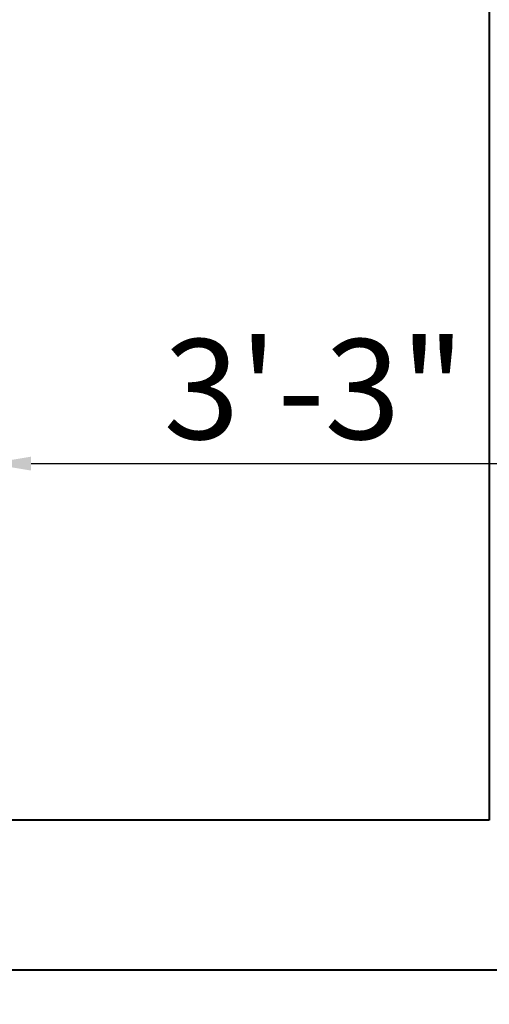
# Model space of a CAD drawing. Units: inches. Extents: x 459864 to 460310, y 324185 to 324787.
# Tile 79 of 112: x 460210 to 460238, y 324281 to 324341. Entities that reach past the tile are written whole.
import ezdxf

# ---------------------------------------------------------------- set-up
doc = ezdxf.new("R2010")
doc.units = ezdxf.units.IN
for name, color, linetype, lineweight in [('A-ANNO-DIMS', 2, 'Continuous', 18), ('A-WALL', 7, 'Continuous', 40), ('L-SITE-PATT', 252, 'Continuous', 13)]:
    doc.layers.add(name, color=color, linetype=linetype, lineweight=lineweight)
doc.styles.get("Standard").update_dxf_attribs({"font": 'arial.ttf'})
doc.dimstyles.new('ISO-25', dxfattribs={"dimtxt": 6, "dimasz": 2.5, "dimexe": 1.25, "dimexo": 0.625, "dimtad": 1, "dimdec": 1, "dimlunit": 3, "dimtxsty": 'Standard', "dimcen": 2.5, "dimadec": 0, "dimazin": 0, "dimtfac": 1, "dimtdec": 1, "dimtmove": 0, "dimatfit": 3, "dimfxl": 1, "dimarcsym": 0})

# ---------------------------------------------------------------- blocks, each defined once
blk = doc.blocks.new('*D67')
at = {"layer": 'A-ANNO-DIMS', "color": 0, "lineweight": -2, "transparency": 16777216}
for p, q in [((460208.115, 324284.108), (460208.115, 324315.133)), ((460247.115, 324284.108), (460247.115, 324315.133)), ((460210.615, 324313.883), (460244.615, 324313.883))]:
    blk.add_line(p, q, dxfattribs=at)
at = {"layer": 'A-ANNO-DIMS', "color": 0, "transparency": 16777216}
for points in [[(460210.615, 324314.3), (460210.615, 324313.467), (460208.115, 324313.883)], [(460244.615, 324314.3), (460244.615, 324313.467), (460247.115, 324313.883)]]:
    blk.add_solid(points, dxfattribs=at)
at = {"layer": 'Defpoints', "color": 0, "transparency": 16777216}
for p in [(460247.115, 324313.883), (460208.115, 324283.483), (460247.115, 324283.483)]:
    blk.add_point(p, dxfattribs=at)
at = {"layer": 'A-ANNO-DIMS', "color": 0, "transparency": 16777216, "insert": (460227.615, 324317.574), "char_height": 6, "attachment_point": 5}
blk.add_mtext('3\'-3"', dxfattribs=at)

msp = doc.modelspace()

# ---------------------------------------------------------------- hatches: boundary and pattern name
at = {"layer": 'L-SITE-PATT'}
h = msp.add_hatch(dxfattribs=at)
h.set_pattern_fill('DOTS', color=256)
h.paths.add_polyline_path([(460269.804, 324283.483), (460247.115, 324283.483), (460121.929, 324283.483), (460121.929, 324252.473), (460117.429, 324252.473), (460110.124, 324252.473), (460110.124, 324243.287), (460080.83, 324243.287), (460080.83, 324252.473), (460061.115, 324252.473), (460061.115, 324251.882), (460077.909, 324251.882), (460077.909, 324199.483), (460080.83, 324199.483), (460080.83, 324207.553), (460110.124, 324207.553), (460110.124, 324199.483), (460110.813, 324199.483), (460262.115, 324199.483), (460269.804, 324199.483)], flags=17)
edge = h.paths.add_edge_path(flags=0)
edge.add_ellipse((460222.59, 324263.813), major_axis=(-8.485, 8.485), ratio=1, start_angle=405, end_angle=495, ccw=False)
edge.add_line((460214.821, 324254.66), (460214.832, 324254.666))
edge.add_ellipse((460222.59, 324263.813), major_axis=(-8.485, 8.485), ratio=1, start_angle=405, end_angle=495, ccw=False)
edge.add_line((460210.759, 324261.781), (460210.768, 324261.787))
edge.add_ellipse((460222.59, 324263.813), major_axis=(-8.485, 8.485), ratio=1, start_angle=405, end_angle=495, ccw=False)
edge.add_ellipse((460222.59, 324263.813), major_axis=(-8.485, 8.485), ratio=1, start_angle=392.75402, end_angle=405, ccw=False)
edge.add_ellipse((460222.59, 324263.813), major_axis=(-8.485, 8.485), ratio=1, start_angle=380.93472, end_angle=392.75402, ccw=False)
edge.add_line((460211.337, 324267.985), (460211.34, 324267.985))
edge.add_ellipse((460222.59, 324263.813), major_axis=(-8.485, 8.485), ratio=1, start_angle=380.93472, end_angle=392.75402, ccw=False)
edge.add_ellipse((460222.59, 324263.813), major_axis=(-8.485, 8.485), ratio=1, start_angle=347.90152, end_angle=380.93472, ccw=False)
edge.add_ellipse((460222.59, 324263.813), major_axis=(-8.485, 8.485), ratio=1, start_angle=327.06192, end_angle=347.90152, ccw=False)
edge.add_ellipse((460222.59, 324263.813), major_axis=(-8.485, 8.485), ratio=1, start_angle=278.32464, end_angle=327.06192, ccw=False)
edge.add_line((460225.158, 324275.536), (460225.158, 324275.535))
edge.add_ellipse((460222.59, 324263.813), major_axis=(-8.485, 8.485), ratio=1, start_angle=278.32464, end_angle=327.06192, ccw=False)
edge.add_ellipse((460222.59, 324263.813), major_axis=(-8.485, 8.485), ratio=1, start_angle=260.64357, end_angle=278.32464, ccw=False)
edge.add_ellipse((460222.59, 324263.813), major_axis=(-8.485, 8.485), ratio=1, start_angle=225, end_angle=260.64357, ccw=False)
edge.add_line((460234.509, 324265.243), (460234.501, 324265.239))
edge.add_ellipse((460222.59, 324263.813), major_axis=(-8.485, 8.485), ratio=1, start_angle=225, end_angle=260.64357, ccw=False)
edge.add_ellipse((460222.59, 324263.813), major_axis=(-8.485, 8.485), ratio=1, start_angle=495, end_angle=585, ccw=False)
edge.add_line((460234.437, 324261.861), (460234.424, 324261.858))
edge.add_ellipse((460222.59, 324263.813), major_axis=(-8.485, 8.485), ratio=1, start_angle=495, end_angle=585, ccw=False)
edge.add_line((460227.95, 324253.067), (460227.946, 324253.083))
edge.add_ellipse((460222.59, 324263.813), major_axis=(-8.485, 8.485), ratio=1, start_angle=495, end_angle=585, ccw=False)
edge.add_line((460226.223, 324252.369), (460226.211, 324252.38))
edge.add_ellipse((460222.59, 324263.813), major_axis=(-8.485, 8.485), ratio=1, start_angle=495, end_angle=585, ccw=False)
h.paths.add_polyline_path([(460219.651, 324254.347), (460218.461, 324253.545), (460218.275, 324254.789), (460219.642, 324256.542), (460219.625, 324260.848), (460216.11, 324257.333), (460214.35, 324256.978), (460215.416, 324259.356), (460212.524, 324258.496), (460213.137, 324259.93), (460218.507, 324263.813), (460222.59, 324263.813), (460222.59, 324267.807), (460218.176, 324272.212), (460219.026, 324274.639), (460222.59, 324272.811), (460222.59, 324275.423), (460223.057, 324274.825), (460222.675, 324273.492), (460225.912, 324267.135), (460219.625, 324260.848)], flags=0)
edge = h.paths.add_edge_path(flags=0)
edge.add_ellipse((460194.576, 324264.046), major_axis=(-8.485, 8.485), ratio=1, start_angle=495, end_angle=585, ccw=False)
edge.add_line((460199.936, 324253.3), (460199.932, 324253.316))
edge.add_ellipse((460194.576, 324264.046), major_axis=(-8.485, 8.485), ratio=1, start_angle=495, end_angle=585, ccw=False)
edge.add_line((460198.208, 324252.603), (460198.196, 324252.613))
edge.add_ellipse((460194.576, 324264.046), major_axis=(-8.485, 8.485), ratio=1, start_angle=495, end_angle=585, ccw=False)
edge.add_ellipse((460194.576, 324264.046), major_axis=(-8.485, 8.485), ratio=1, start_angle=405, end_angle=495, ccw=False)
edge.add_line((460186.806, 324254.893), (460186.817, 324254.899))
edge.add_ellipse((460194.576, 324264.046), major_axis=(-8.485, 8.485), ratio=1, start_angle=405, end_angle=495, ccw=False)
edge.add_line((460182.744, 324262.014), (460182.753, 324262.02))
edge.add_ellipse((460194.576, 324264.046), major_axis=(-8.485, 8.485), ratio=1, start_angle=405, end_angle=495, ccw=False)
edge.add_ellipse((460194.576, 324264.046), major_axis=(-8.485, 8.485), ratio=1, start_angle=392.75402, end_angle=405, ccw=False)
edge.add_ellipse((460194.576, 324264.046), major_axis=(-8.485, 8.485), ratio=1, start_angle=380.93472, end_angle=392.75402, ccw=False)
edge.add_line((460183.323, 324268.218), (460183.326, 324268.218))
edge.add_ellipse((460194.576, 324264.046), major_axis=(-8.485, 8.485), ratio=1, start_angle=380.93472, end_angle=392.75402, ccw=False)
edge.add_ellipse((460194.576, 324264.046), major_axis=(-8.485, 8.485), ratio=1, start_angle=347.90152, end_angle=380.93472, ccw=False)
edge.add_ellipse((460194.576, 324264.046), major_axis=(-8.485, 8.485), ratio=1, start_angle=327.06192, end_angle=347.90152, ccw=False)
edge.add_ellipse((460194.576, 324264.046), major_axis=(-8.485, 8.485), ratio=1, start_angle=278.32464, end_angle=327.06192, ccw=False)
edge.add_line((460197.144, 324275.769), (460197.143, 324275.768))
edge.add_ellipse((460194.576, 324264.046), major_axis=(-8.485, 8.485), ratio=1, start_angle=278.32464, end_angle=327.06192, ccw=False)
edge.add_ellipse((460194.576, 324264.046), major_axis=(-8.485, 8.485), ratio=1, start_angle=260.64357, end_angle=278.32464, ccw=False)
edge.add_ellipse((460194.576, 324264.046), major_axis=(-8.485, 8.485), ratio=1, start_angle=225, end_angle=260.64357, ccw=False)
edge.add_line((460206.494, 324265.476), (460206.487, 324265.473))
edge.add_ellipse((460194.576, 324264.046), major_axis=(-8.485, 8.485), ratio=1, start_angle=225, end_angle=260.64357, ccw=False)
edge.add_ellipse((460194.576, 324264.046), major_axis=(-8.485, 8.485), ratio=1, start_angle=495, end_angle=585, ccw=False)
edge.add_line((460206.422, 324262.094), (460206.409, 324262.091))
h.paths.add_polyline_path([(460191.61, 324261.081), (460191.637, 324254.58), (460190.447, 324253.778), (460190.261, 324255.023), (460191.628, 324256.775), (460191.61, 324261.081), (460188.096, 324257.566), (460186.335, 324257.211), (460187.402, 324259.589), (460184.509, 324258.729), (460185.123, 324260.163), (460190.493, 324264.046), (460194.576, 324264.046), (460194.576, 324268.04), (460190.161, 324272.446), (460191.011, 324274.872), (460194.576, 324273.044), (460194.576, 324275.657), (460195.043, 324275.058), (460194.661, 324273.725), (460197.897, 324267.368)], flags=0)
edge = h.paths.add_edge_path(flags=0)
edge.add_ellipse((460252.912, 324263.578), major_axis=(-8.485, 8.485), ratio=1, start_angle=405, end_angle=495, ccw=False)
edge.add_line((460241.081, 324261.545), (460241.089, 324261.551))
edge.add_ellipse((460252.912, 324263.578), major_axis=(-8.485, 8.485), ratio=1, start_angle=405, end_angle=495, ccw=False)
edge.add_ellipse((460252.912, 324263.578), major_axis=(-8.485, 8.485), ratio=1, start_angle=392.75402, end_angle=405, ccw=False)
edge.add_ellipse((460252.912, 324263.578), major_axis=(-8.485, 8.485), ratio=1, start_angle=380.93472, end_angle=392.75402, ccw=False)
edge.add_line((460241.659, 324267.749), (460241.662, 324267.749))
edge.add_ellipse((460252.912, 324263.578), major_axis=(-8.485, 8.485), ratio=1, start_angle=380.93472, end_angle=392.75402, ccw=False)
edge.add_ellipse((460252.912, 324263.578), major_axis=(-8.485, 8.485), ratio=1, start_angle=347.90152, end_angle=380.93472, ccw=False)
edge.add_ellipse((460252.912, 324263.578), major_axis=(-8.485, 8.485), ratio=1, start_angle=327.06192, end_angle=347.90152, ccw=False)
edge.add_ellipse((460252.912, 324263.578), major_axis=(-8.485, 8.485), ratio=1, start_angle=278.32464, end_angle=327.06192, ccw=False)
edge.add_line((460255.48, 324275.3), (460255.479, 324275.299))
edge.add_ellipse((460252.912, 324263.578), major_axis=(-8.485, 8.485), ratio=1, start_angle=278.32464, end_angle=327.06192, ccw=False)
edge.add_ellipse((460252.912, 324263.578), major_axis=(-8.485, 8.485), ratio=1, start_angle=260.64357, end_angle=278.32464, ccw=False)
edge.add_ellipse((460252.912, 324263.578), major_axis=(-8.485, 8.485), ratio=1, start_angle=225, end_angle=260.64357, ccw=False)
edge.add_line((460264.83, 324265.007), (460264.823, 324265.004))
edge.add_ellipse((460252.912, 324263.578), major_axis=(-8.485, 8.485), ratio=1, start_angle=225, end_angle=260.64357, ccw=False)
edge.add_ellipse((460252.912, 324263.578), major_axis=(-8.485, 8.485), ratio=1, start_angle=495, end_angle=585, ccw=False)
edge.add_line((460264.758, 324261.626), (460264.745, 324261.622))
edge.add_ellipse((460252.912, 324263.578), major_axis=(-8.485, 8.485), ratio=1, start_angle=495, end_angle=585, ccw=False)
edge.add_line((460258.272, 324252.832), (460258.268, 324252.848))
edge.add_ellipse((460252.912, 324263.578), major_axis=(-8.485, 8.485), ratio=1, start_angle=495, end_angle=585, ccw=False)
edge.add_line((460256.545, 324252.134), (460256.533, 324252.144))
edge.add_ellipse((460252.912, 324263.578), major_axis=(-8.485, 8.485), ratio=1, start_angle=495, end_angle=585, ccw=False)
edge.add_ellipse((460252.912, 324263.578), major_axis=(-8.485, 8.485), ratio=1, start_angle=405, end_angle=495, ccw=False)
edge.add_line((460245.143, 324254.424), (460245.153, 324254.43))
h.paths.add_polyline_path([(460244.672, 324256.742), (460245.738, 324259.12), (460242.846, 324258.26), (460243.459, 324259.694), (460248.829, 324263.578), (460252.912, 324263.578), (460252.912, 324267.571), (460248.497, 324271.977), (460249.348, 324274.403), (460252.912, 324272.576), (460252.912, 324275.188), (460253.379, 324274.589), (460252.997, 324273.257), (460256.233, 324266.899), (460249.946, 324260.612), (460249.973, 324254.111), (460248.783, 324253.309), (460248.597, 324254.554), (460249.964, 324256.306), (460249.946, 324260.612), (460246.432, 324257.097)], flags=0)
edge = h.paths.add_edge_path(flags=0)
edge.add_ellipse((460167.439, 324262.833), major_axis=(-8.485, 8.485), ratio=1, start_angle=495, end_angle=585, ccw=False)
edge.add_line((460172.799, 324252.087), (460172.795, 324252.103))
edge.add_ellipse((460167.439, 324262.833), major_axis=(-8.485, 8.485), ratio=1, start_angle=495, end_angle=585, ccw=False)
edge.add_line((460171.071, 324251.389), (460171.059, 324251.399))
edge.add_ellipse((460167.439, 324262.833), major_axis=(-8.485, 8.485), ratio=1, start_angle=495, end_angle=585, ccw=False)
edge.add_ellipse((460167.439, 324262.833), major_axis=(-8.485, 8.485), ratio=1, start_angle=405, end_angle=495, ccw=False)
edge.add_line((460159.669, 324253.679), (460159.68, 324253.685))
edge.add_ellipse((460167.439, 324262.833), major_axis=(-8.485, 8.485), ratio=1, start_angle=405, end_angle=495, ccw=False)
edge.add_line((460155.607, 324260.8), (460155.616, 324260.806))
edge.add_ellipse((460167.439, 324262.833), major_axis=(-8.485, 8.485), ratio=1, start_angle=405, end_angle=495, ccw=False)
edge.add_ellipse((460167.439, 324262.833), major_axis=(-8.485, 8.485), ratio=1, start_angle=392.75402, end_angle=405, ccw=False)
edge.add_ellipse((460167.439, 324262.833), major_axis=(-8.485, 8.485), ratio=1, start_angle=380.93472, end_angle=392.75402, ccw=False)
edge.add_line((460156.185, 324267.005), (460156.189, 324267.005))
edge.add_ellipse((460167.439, 324262.833), major_axis=(-8.485, 8.485), ratio=1, start_angle=380.93472, end_angle=392.75402, ccw=False)
edge.add_ellipse((460167.439, 324262.833), major_axis=(-8.485, 8.485), ratio=1, start_angle=347.90152, end_angle=380.93472, ccw=False)
edge.add_ellipse((460167.439, 324262.833), major_axis=(-8.485, 8.485), ratio=1, start_angle=327.06192, end_angle=347.90152, ccw=False)
edge.add_ellipse((460167.439, 324262.833), major_axis=(-8.485, 8.485), ratio=1, start_angle=278.32464, end_angle=327.06192, ccw=False)
edge.add_line((460170.007, 324274.556), (460170.006, 324274.554))
edge.add_ellipse((460167.439, 324262.833), major_axis=(-8.485, 8.485), ratio=1, start_angle=278.32464, end_angle=327.06192, ccw=False)
edge.add_ellipse((460167.439, 324262.833), major_axis=(-8.485, 8.485), ratio=1, start_angle=260.64357, end_angle=278.32464, ccw=False)
edge.add_ellipse((460167.439, 324262.833), major_axis=(-8.485, 8.485), ratio=1, start_angle=225, end_angle=260.64357, ccw=False)
edge.add_line((460179.357, 324264.262), (460179.35, 324264.259))
edge.add_ellipse((460167.439, 324262.833), major_axis=(-8.485, 8.485), ratio=1, start_angle=225, end_angle=260.64357, ccw=False)
edge.add_ellipse((460167.439, 324262.833), major_axis=(-8.485, 8.485), ratio=1, start_angle=495, end_angle=585, ccw=False)
edge.add_line((460179.285, 324260.881), (460179.272, 324260.877))
h.paths.add_polyline_path([(460164.473, 324259.867), (460164.5, 324253.366), (460163.31, 324252.565), (460163.124, 324253.809), (460164.491, 324255.561), (460164.473, 324259.867), (460160.958, 324256.353), (460159.198, 324255.998), (460160.265, 324258.375), (460157.372, 324257.515), (460157.986, 324258.949), (460163.356, 324262.833), (460167.439, 324262.833), (460167.439, 324266.826), (460163.024, 324271.232), (460163.874, 324273.659), (460167.439, 324271.831), (460167.439, 324274.443), (460167.905, 324273.844), (460167.524, 324272.512), (460170.76, 324266.154)], flags=0)
edge = h.paths.add_edge_path(flags=0)
edge.add_ellipse((460140.758, 324262.37), major_axis=(-8.485, 8.485), ratio=1, start_angle=495, end_angle=585, ccw=False)
edge.add_line((460146.118, 324251.624), (460146.114, 324251.639))
edge.add_ellipse((460140.758, 324262.37), major_axis=(-8.485, 8.485), ratio=1, start_angle=495, end_angle=585, ccw=False)
edge.add_line((460144.391, 324250.926), (460144.379, 324250.936))
edge.add_ellipse((460140.758, 324262.37), major_axis=(-8.485, 8.485), ratio=1, start_angle=495, end_angle=585, ccw=False)
edge.add_ellipse((460140.758, 324262.37), major_axis=(-8.485, 8.485), ratio=1, start_angle=405, end_angle=495, ccw=False)
edge.add_line((460132.989, 324253.216), (460132.999, 324253.222))
edge.add_ellipse((460140.758, 324262.37), major_axis=(-8.485, 8.485), ratio=1, start_angle=405, end_angle=495, ccw=False)
edge.add_line((460128.927, 324260.337), (460128.935, 324260.343))
edge.add_ellipse((460140.758, 324262.37), major_axis=(-8.485, 8.485), ratio=1, start_angle=405, end_angle=495, ccw=False)
edge.add_ellipse((460140.758, 324262.37), major_axis=(-8.485, 8.485), ratio=1, start_angle=392.75402, end_angle=405, ccw=False)
edge.add_ellipse((460140.758, 324262.37), major_axis=(-8.485, 8.485), ratio=1, start_angle=380.93472, end_angle=392.75402, ccw=False)
edge.add_line((460129.505, 324266.541), (460129.508, 324266.541))
edge.add_ellipse((460140.758, 324262.37), major_axis=(-8.485, 8.485), ratio=1, start_angle=380.93472, end_angle=392.75402, ccw=False)
edge.add_ellipse((460140.758, 324262.37), major_axis=(-8.485, 8.485), ratio=1, start_angle=347.90152, end_angle=380.93472, ccw=False)
edge.add_ellipse((460140.758, 324262.37), major_axis=(-8.485, 8.485), ratio=1, start_angle=327.06192, end_angle=347.90152, ccw=False)
edge.add_ellipse((460140.758, 324262.37), major_axis=(-8.485, 8.485), ratio=1, start_angle=278.32464, end_angle=327.06192, ccw=False)
edge.add_line((460143.326, 324274.092), (460143.325, 324274.091))
edge.add_ellipse((460140.758, 324262.37), major_axis=(-8.485, 8.485), ratio=1, start_angle=278.32464, end_angle=327.06192, ccw=False)
edge.add_ellipse((460140.758, 324262.37), major_axis=(-8.485, 8.485), ratio=1, start_angle=260.64357, end_angle=278.32464, ccw=False)
edge.add_ellipse((460140.758, 324262.37), major_axis=(-8.485, 8.485), ratio=1, start_angle=225, end_angle=260.64357, ccw=False)
edge.add_line((460152.677, 324263.799), (460152.669, 324263.796))
edge.add_ellipse((460140.758, 324262.37), major_axis=(-8.485, 8.485), ratio=1, start_angle=225, end_angle=260.64357, ccw=False)
edge.add_ellipse((460140.758, 324262.37), major_axis=(-8.485, 8.485), ratio=1, start_angle=495, end_angle=585, ccw=False)
edge.add_line((460152.604, 324260.418), (460152.592, 324260.414))
h.paths.add_polyline_path([(460137.792, 324259.404), (460137.819, 324252.903), (460136.629, 324252.101), (460136.443, 324253.346), (460137.81, 324255.098), (460137.792, 324259.404), (460134.278, 324255.889), (460132.518, 324255.534), (460133.584, 324257.912), (460130.692, 324257.052), (460131.305, 324258.486), (460136.675, 324262.37), (460140.758, 324262.37), (460140.758, 324266.363), (460136.343, 324270.769), (460137.194, 324273.195), (460140.758, 324271.367), (460140.758, 324273.98), (460141.225, 324273.381), (460140.843, 324272.049), (460144.079, 324265.691)], flags=0)
h.paths.add_polyline_path([(460110.124, 324227.414), (460080.83, 324227.414), (460080.83, 324235.484), (460110.124, 324235.484)], flags=16)
h.paths.add_polyline_path([(460110.124, 324220.797), (460110.124, 324212.727), (460080.83, 324212.727), (460080.83, 324220.797)], flags=16)
h.paths.add_polyline_path([(460269.804, 324283.483), (460247.115, 324283.483), (460121.929, 324283.483), (460121.929, 324252.473), (460117.429, 324252.473), (460110.124, 324252.473), (460110.124, 324243.287), (460080.83, 324243.287), (460080.83, 324252.473), (460061.115, 324252.473), (460061.115, 324251.882), (460077.909, 324251.882), (460077.909, 324199.483), (460080.83, 324199.483), (460080.83, 324207.553), (460110.124, 324207.553), (460110.124, 324199.483), (460262.115, 324199.483), (460269.804, 324199.483)], flags=17)
h.paths.add_polyline_path([(460219.651, 324254.347), (460218.461, 324253.545), (460218.275, 324254.789), (460219.642, 324256.542), (460219.625, 324260.848), (460216.11, 324257.333), (460214.35, 324256.978), (460215.416, 324259.356), (460212.524, 324258.496), (460213.137, 324259.93), (460218.507, 324263.813), (460222.59, 324263.813), (460220.18, 324266.223), (460215.461, 324265.308), (460211.835, 324266.137), (460216.247, 324267.985), (460218.418, 324267.985), (460222.59, 324263.813), (460222.59, 324267.807), (460218.176, 324272.212), (460219.026, 324274.639), (460222.59, 324272.811), (460222.59, 324275.423), (460223.057, 324274.825), (460222.675, 324273.492), (460225.912, 324267.135), (460222.59, 324263.813), (460231.383, 324263.813), (460228.485, 324262.488), (460224.425, 324261.978), (460228.68, 324257.724), (460228.966, 324254.791), (460227.142, 324256.537), (460227.542, 324254.819), (460227.333, 324253.614), (460222.59, 324259.985), (460222.59, 324255.497), (460221.377, 324256.541), (460220.576, 324261.799), (460219.625, 324260.848)], flags=0)
h.paths.add_polyline_path([(460199.127, 324256.77), (460199.528, 324255.052), (460199.319, 324253.848), (460194.576, 324260.218), (460194.576, 324255.73), (460193.363, 324256.774), (460192.561, 324262.032), (460191.61, 324261.081), (460191.637, 324254.58), (460190.447, 324253.778), (460190.261, 324255.023), (460191.628, 324256.775), (460191.61, 324261.081), (460188.096, 324257.566), (460186.335, 324257.211), (460187.402, 324259.589), (460184.509, 324258.729), (460185.123, 324260.163), (460190.493, 324264.046), (460194.576, 324264.046), (460192.166, 324266.456), (460187.446, 324265.541), (460183.82, 324266.37), (460188.232, 324268.218), (460190.404, 324268.218), (460194.576, 324264.046), (460194.576, 324268.04), (460190.161, 324272.446), (460191.011, 324274.872), (460194.576, 324273.044), (460194.576, 324275.657), (460195.043, 324275.058), (460194.661, 324273.725), (460197.897, 324267.368), (460194.576, 324264.046), (460203.368, 324264.046), (460200.47, 324262.721), (460196.411, 324262.212), (460200.665, 324257.957), (460200.951, 324255.024)], flags=0)
h.paths.add_polyline_path([(460244.672, 324256.742), (460245.738, 324259.12), (460242.846, 324258.26), (460243.459, 324259.694), (460248.829, 324263.578), (460252.912, 324263.578), (460250.502, 324265.987), (460245.783, 324265.072), (460242.156, 324265.901), (460246.568, 324267.749), (460248.74, 324267.749), (460252.912, 324263.578), (460252.912, 324267.571), (460248.497, 324271.977), (460249.348, 324274.403), (460252.912, 324272.576), (460252.912, 324275.188), (460253.379, 324274.589), (460252.997, 324273.257), (460256.233, 324266.899), (460252.912, 324263.578), (460261.705, 324263.578), (460258.806, 324262.252), (460254.747, 324261.743), (460259.002, 324257.488), (460259.288, 324254.555), (460257.463, 324256.301), (460257.864, 324254.583), (460257.655, 324253.379), (460252.912, 324259.749), (460252.912, 324255.261), (460251.699, 324256.305), (460250.897, 324261.563), (460249.946, 324260.612), (460249.973, 324254.111), (460248.783, 324253.309), (460248.597, 324254.554), (460249.964, 324256.306), (460249.946, 324260.612), (460246.432, 324257.097)], flags=0)
h.paths.add_polyline_path([(460173.528, 324256.743), (460173.814, 324253.811), (460171.99, 324255.556), (460172.39, 324253.838), (460172.182, 324252.634), (460167.439, 324259.004), (460167.439, 324254.516), (460166.226, 324255.56), (460165.424, 324260.818), (460164.473, 324259.867), (460164.5, 324253.366), (460163.31, 324252.565), (460163.124, 324253.809), (460164.491, 324255.561), (460164.473, 324259.867), (460160.958, 324256.353), (460159.198, 324255.998), (460160.265, 324258.375), (460157.372, 324257.515), (460157.986, 324258.949), (460163.356, 324262.833), (460167.439, 324262.833), (460165.029, 324265.243), (460160.309, 324264.327), (460156.683, 324265.156), (460161.095, 324267.005), (460163.267, 324267.005), (460167.439, 324262.833), (460167.439, 324266.826), (460163.024, 324271.232), (460163.874, 324273.659), (460167.439, 324271.831), (460167.439, 324274.443), (460167.905, 324273.844), (460167.524, 324272.512), (460170.76, 324266.154), (460167.439, 324262.833), (460176.231, 324262.833), (460173.333, 324261.507), (460169.274, 324260.998)], flags=0)
h.paths.add_polyline_path([(460146.848, 324256.28), (460147.134, 324253.347), (460145.31, 324255.093), (460145.71, 324253.375), (460145.501, 324252.171), (460140.758, 324258.541), (460140.758, 324254.053), (460139.545, 324255.097), (460138.744, 324260.355), (460137.792, 324259.404), (460137.819, 324252.903), (460136.629, 324252.101), (460136.443, 324253.346), (460137.81, 324255.098), (460137.792, 324259.404), (460134.278, 324255.889), (460132.518, 324255.534), (460133.584, 324257.912), (460130.692, 324257.052), (460131.305, 324258.486), (460136.675, 324262.37), (460140.758, 324262.37), (460138.348, 324264.779), (460133.629, 324263.864), (460130.002, 324264.693), (460134.414, 324266.541), (460136.586, 324266.541), (460140.758, 324262.37), (460140.758, 324266.363), (460136.343, 324270.769), (460137.194, 324273.195), (460140.758, 324271.367), (460140.758, 324273.98), (460141.225, 324273.381), (460140.843, 324272.049), (460144.079, 324265.691), (460140.758, 324262.37), (460149.551, 324262.37), (460146.653, 324261.044), (460142.593, 324260.535)], flags=0)
edge = h.paths.add_edge_path()
edge.add_line((460269.804, 324272.549), (460260.881, 324272.549))
edge.add_ellipse((460252.912, 324263.578), major_axis=(-8.485, 8.485), ratio=1, start_angle=260.64357, end_angle=273.38462, ccw=False)
edge.add_line((460262.283, 324271.092), (460262.261, 324271.091))
edge.add_ellipse((460252.912, 324263.578), major_axis=(-8.485, 8.485), ratio=1, start_angle=260.64357, end_angle=273.38462, ccw=False)
edge.add_ellipse((460252.912, 324263.578), major_axis=(-8.485, 8.485), ratio=1, start_angle=225, end_angle=260.64357, ccw=False)
edge.add_line((460263.609, 324269.063), (460263.572, 324269.058))
edge.add_ellipse((460252.912, 324263.578), major_axis=(-8.485, 8.485), ratio=1, start_angle=225, end_angle=260.64357, ccw=False)
edge.add_line((460264.615, 324266.306), (460264.585, 324266.305))
edge.add_ellipse((460252.912, 324263.578), major_axis=(-8.485, 8.485), ratio=1, start_angle=225, end_angle=260.64357, ccw=False)
edge.add_line((460264.83, 324265.007), (460264.823, 324265.004))
edge.add_ellipse((460252.912, 324263.578), major_axis=(-8.485, 8.485), ratio=1, start_angle=225, end_angle=260.64357, ccw=False)
edge.add_ellipse((460252.912, 324263.578), major_axis=(-8.485, 8.485), ratio=1, start_angle=495, end_angle=585, ccw=False)
edge.add_line((460264.758, 324261.626), (460264.745, 324261.622))
edge.add_ellipse((460252.912, 324263.578), major_axis=(-8.485, 8.485), ratio=1, start_angle=495, end_angle=585, ccw=False)
edge.add_line((460263.442, 324257.739), (460263.389, 324257.779))
edge.add_ellipse((460252.912, 324263.578), major_axis=(-8.485, 8.485), ratio=1, start_angle=495, end_angle=585, ccw=False)
edge.add_line((460258.128, 324252.744), (460258.102, 324252.779))
edge.add_ellipse((460252.912, 324263.578), major_axis=(-8.485, 8.485), ratio=1, start_angle=495, end_angle=585, ccw=False)
edge.add_line((460256.545, 324252.134), (460256.533, 324252.144))
edge.add_ellipse((460252.912, 324263.578), major_axis=(-8.485, 8.485), ratio=1, start_angle=495, end_angle=585, ccw=False)
edge.add_ellipse((460252.912, 324263.578), major_axis=(-8.485, 8.485), ratio=1, start_angle=405, end_angle=495, ccw=False)
edge.add_line((460250.594, 324251.78), (460250.605, 324251.82))
edge.add_ellipse((460252.912, 324263.578), major_axis=(-8.485, 8.485), ratio=1, start_angle=405, end_angle=495, ccw=False)
edge.add_line((460245.143, 324254.424), (460245.153, 324254.43))
edge.add_ellipse((460252.912, 324263.578), major_axis=(-8.485, 8.485), ratio=1, start_angle=405, end_angle=495, ccw=False)
edge.add_line((460243.525, 324256.059), (460243.56, 324256.091))
edge.add_ellipse((460252.912, 324263.578), major_axis=(-8.485, 8.485), ratio=1, start_angle=405, end_angle=495, ccw=False)
edge.add_line((460241.44, 324259.893), (460241.522, 324259.896))
edge.add_ellipse((460252.912, 324263.578), major_axis=(-8.485, 8.485), ratio=1, start_angle=405, end_angle=495, ccw=False)
edge.add_line((460241.081, 324261.545), (460241.089, 324261.551))
edge.add_ellipse((460252.912, 324263.578), major_axis=(-8.485, 8.485), ratio=1, start_angle=405, end_angle=495, ccw=False)
edge.add_ellipse((460252.912, 324263.578), major_axis=(-8.485, 8.485), ratio=1, start_angle=392.75402, end_angle=405, ccw=False)
edge.add_line((460241.05, 324265.438), (460241.063, 324265.443))
edge.add_ellipse((460252.912, 324263.578), major_axis=(-8.485, 8.485), ratio=1, start_angle=392.75402, end_angle=405, ccw=False)
edge.add_ellipse((460252.912, 324263.578), major_axis=(-8.485, 8.485), ratio=1, start_angle=380.93472, end_angle=392.75402, ccw=False)
edge.add_line((460241.452, 324267.176), (460241.469, 324267.171))
edge.add_ellipse((460252.912, 324263.578), major_axis=(-8.485, 8.485), ratio=1, start_angle=380.93472, end_angle=392.75402, ccw=False)
edge.add_line((460241.659, 324267.749), (460241.662, 324267.749))
edge.add_ellipse((460252.912, 324263.578), major_axis=(-8.485, 8.485), ratio=1, start_angle=380.93472, end_angle=392.75402, ccw=False)
edge.add_ellipse((460252.912, 324263.578), major_axis=(-8.485, 8.485), ratio=1, start_angle=356.61538, end_angle=380.93472, ccw=False)
edge.add_line((460244.88, 324272.488), (460244.713, 324272.549))
edge.add_line((460244.713, 324272.549), (460230.817, 324272.549))
edge.add_ellipse((460222.59, 324263.813), major_axis=(-8.485, 8.485), ratio=1, start_angle=260.64357, end_angle=271.71777, ccw=False)
edge.add_ellipse((460222.59, 324263.813), major_axis=(-8.485, 8.485), ratio=1, start_angle=225, end_angle=260.64357, ccw=False)
edge.add_line((460233.287, 324269.299), (460233.25, 324269.294))
edge.add_ellipse((460222.59, 324263.813), major_axis=(-8.485, 8.485), ratio=1, start_angle=225, end_angle=260.64357, ccw=False)
edge.add_line((460234.294, 324266.541), (460234.264, 324266.541))
edge.add_ellipse((460222.59, 324263.813), major_axis=(-8.485, 8.485), ratio=1, start_angle=225, end_angle=260.64357, ccw=False)
edge.add_line((460234.509, 324265.243), (460234.501, 324265.239))
edge.add_ellipse((460222.59, 324263.813), major_axis=(-8.485, 8.485), ratio=1, start_angle=225, end_angle=260.64357, ccw=False)
edge.add_ellipse((460222.59, 324263.813), major_axis=(-8.485, 8.485), ratio=1, start_angle=495, end_angle=585, ccw=False)
edge.add_line((460234.437, 324261.861), (460234.424, 324261.858))
edge.add_ellipse((460222.59, 324263.813), major_axis=(-8.485, 8.485), ratio=1, start_angle=495, end_angle=585, ccw=False)
edge.add_line((460233.121, 324257.975), (460233.068, 324258.015))
edge.add_ellipse((460222.59, 324263.813), major_axis=(-8.485, 8.485), ratio=1, start_angle=495, end_angle=585, ccw=False)
edge.add_line((460227.806, 324252.979), (460227.78, 324253.014))
edge.add_ellipse((460222.59, 324263.813), major_axis=(-8.485, 8.485), ratio=1, start_angle=495, end_angle=585, ccw=False)
edge.add_line((460226.223, 324252.369), (460226.211, 324252.38))
edge.add_ellipse((460222.59, 324263.813), major_axis=(-8.485, 8.485), ratio=1, start_angle=495, end_angle=585, ccw=False)
edge.add_ellipse((460222.59, 324263.813), major_axis=(-8.485, 8.485), ratio=1, start_angle=405, end_angle=495, ccw=False)
edge.add_line((460220.272, 324252.016), (460220.283, 324252.055))
edge.add_ellipse((460222.59, 324263.813), major_axis=(-8.485, 8.485), ratio=1, start_angle=405, end_angle=495, ccw=False)
edge.add_line((460214.821, 324254.66), (460214.832, 324254.666))
edge.add_ellipse((460222.59, 324263.813), major_axis=(-8.485, 8.485), ratio=1, start_angle=405, end_angle=495, ccw=False)
edge.add_line((460213.203, 324256.295), (460213.239, 324256.327))
edge.add_ellipse((460222.59, 324263.813), major_axis=(-8.485, 8.485), ratio=1, start_angle=405, end_angle=495, ccw=False)
edge.add_line((460211.118, 324260.128), (460211.201, 324260.131))
edge.add_ellipse((460222.59, 324263.813), major_axis=(-8.485, 8.485), ratio=1, start_angle=405, end_angle=495, ccw=False)
edge.add_line((460210.759, 324261.781), (460210.768, 324261.787))
edge.add_ellipse((460222.59, 324263.813), major_axis=(-8.485, 8.485), ratio=1, start_angle=405, end_angle=495, ccw=False)
edge.add_ellipse((460222.59, 324263.813), major_axis=(-8.485, 8.485), ratio=1, start_angle=392.75402, end_angle=405, ccw=False)
edge.add_line((460210.729, 324265.673), (460210.741, 324265.678))
edge.add_ellipse((460222.59, 324263.813), major_axis=(-8.485, 8.485), ratio=1, start_angle=392.75402, end_angle=405, ccw=False)
edge.add_ellipse((460222.59, 324263.813), major_axis=(-8.485, 8.485), ratio=1, start_angle=380.93472, end_angle=392.75402, ccw=False)
edge.add_line((460211.13, 324267.412), (460211.147, 324267.407))
edge.add_ellipse((460222.59, 324263.813), major_axis=(-8.485, 8.485), ratio=1, start_angle=380.93472, end_angle=392.75402, ccw=False)
edge.add_line((460211.337, 324267.985), (460211.34, 324267.985))
edge.add_ellipse((460222.59, 324263.813), major_axis=(-8.485, 8.485), ratio=1, start_angle=380.93472, end_angle=392.75402, ccw=False)
edge.add_ellipse((460222.59, 324263.813), major_axis=(-8.485, 8.485), ratio=1, start_angle=358.28223, end_angle=380.93472, ccw=False)
edge.add_line((460213.705, 324271.902), (460213.709, 324271.869))
edge.add_ellipse((460222.59, 324263.813), major_axis=(-8.485, 8.485), ratio=1, start_angle=358.28223, end_angle=380.93472, ccw=False)
edge.add_line((460214.363, 324272.549), (460203.078, 324272.549))
edge.add_line((460203.078, 324272.549), (460203.06, 324272.531))
edge.add_ellipse((460194.576, 324264.046), major_axis=(-8.485, 8.485), ratio=1, start_angle=260.64357, end_angle=270.11679, ccw=False)
edge.add_line((460203.957, 324271.561), (460203.921, 324271.56))
edge.add_ellipse((460194.576, 324264.046), major_axis=(-8.485, 8.485), ratio=1, start_angle=260.64357, end_angle=270.11679, ccw=False)
edge.add_ellipse((460194.576, 324264.046), major_axis=(-8.485, 8.485), ratio=1, start_angle=225, end_angle=260.64357, ccw=False)
edge.add_line((460205.272, 324269.532), (460205.235, 324269.527))
edge.add_ellipse((460194.576, 324264.046), major_axis=(-8.485, 8.485), ratio=1, start_angle=225, end_angle=260.64357, ccw=False)
edge.add_line((460206.279, 324266.774), (460206.249, 324266.774))
edge.add_ellipse((460194.576, 324264.046), major_axis=(-8.485, 8.485), ratio=1, start_angle=225, end_angle=260.64357, ccw=False)
edge.add_line((460206.494, 324265.476), (460206.487, 324265.473))
edge.add_ellipse((460194.576, 324264.046), major_axis=(-8.485, 8.485), ratio=1, start_angle=225, end_angle=260.64357, ccw=False)
edge.add_ellipse((460194.576, 324264.046), major_axis=(-8.485, 8.485), ratio=1, start_angle=495, end_angle=585, ccw=False)
edge.add_line((460206.422, 324262.094), (460206.409, 324262.091))
edge.add_ellipse((460194.576, 324264.046), major_axis=(-8.485, 8.485), ratio=1, start_angle=495, end_angle=585, ccw=False)
edge.add_line((460205.106, 324258.208), (460205.053, 324258.248))
edge.add_ellipse((460194.576, 324264.046), major_axis=(-8.485, 8.485), ratio=1, start_angle=495, end_angle=585, ccw=False)
edge.add_line((460199.792, 324253.212), (460199.766, 324253.248))
edge.add_ellipse((460194.576, 324264.046), major_axis=(-8.485, 8.485), ratio=1, start_angle=495, end_angle=585, ccw=False)
edge.add_line((460198.208, 324252.603), (460198.196, 324252.613))
edge.add_ellipse((460194.576, 324264.046), major_axis=(-8.485, 8.485), ratio=1, start_angle=495, end_angle=585, ccw=False)
edge.add_ellipse((460194.576, 324264.046), major_axis=(-8.485, 8.485), ratio=1, start_angle=405, end_angle=495, ccw=False)
edge.add_line((460192.258, 324252.249), (460192.268, 324252.289))
edge.add_ellipse((460194.576, 324264.046), major_axis=(-8.485, 8.485), ratio=1, start_angle=405, end_angle=495, ccw=False)
edge.add_line((460186.806, 324254.893), (460186.817, 324254.899))
edge.add_ellipse((460194.576, 324264.046), major_axis=(-8.485, 8.485), ratio=1, start_angle=405, end_angle=495, ccw=False)
edge.add_line((460185.188, 324256.528), (460185.224, 324256.56))
edge.add_ellipse((460194.576, 324264.046), major_axis=(-8.485, 8.485), ratio=1, start_angle=405, end_angle=495, ccw=False)
edge.add_line((460183.104, 324260.362), (460183.186, 324260.365))
edge.add_ellipse((460194.576, 324264.046), major_axis=(-8.485, 8.485), ratio=1, start_angle=405, end_angle=495, ccw=False)
edge.add_line((460182.744, 324262.014), (460182.753, 324262.02))
edge.add_ellipse((460194.576, 324264.046), major_axis=(-8.485, 8.485), ratio=1, start_angle=405, end_angle=495, ccw=False)
edge.add_ellipse((460194.576, 324264.046), major_axis=(-8.485, 8.485), ratio=1, start_angle=392.75402, end_angle=405, ccw=False)
edge.add_line((460182.714, 324265.906), (460182.726, 324265.912))
edge.add_ellipse((460194.576, 324264.046), major_axis=(-8.485, 8.485), ratio=1, start_angle=392.75402, end_angle=405, ccw=False)
edge.add_ellipse((460194.576, 324264.046), major_axis=(-8.485, 8.485), ratio=1, start_angle=380.93472, end_angle=392.75402, ccw=False)
edge.add_line((460183.116, 324267.645), (460183.133, 324267.64))
edge.add_ellipse((460194.576, 324264.046), major_axis=(-8.485, 8.485), ratio=1, start_angle=380.93472, end_angle=392.75402, ccw=False)
edge.add_line((460183.323, 324268.218), (460183.326, 324268.218))
edge.add_ellipse((460194.576, 324264.046), major_axis=(-8.485, 8.485), ratio=1, start_angle=380.93472, end_angle=392.75402, ccw=False)
edge.add_ellipse((460194.576, 324264.046), major_axis=(-8.485, 8.485), ratio=1, start_angle=359.88321, end_angle=380.93472, ccw=False)
edge.add_line((460184.491, 324270.611), (460184.553, 324270.611))
edge.add_ellipse((460194.576, 324264.046), major_axis=(-8.485, 8.485), ratio=1, start_angle=359.88321, end_angle=380.93472, ccw=False)
edge.add_line((460185.346, 324271.76), (460185.379, 324271.728))
edge.add_ellipse((460194.576, 324264.046), major_axis=(-8.485, 8.485), ratio=1, start_angle=359.88321, end_angle=380.93472, ccw=False)
edge.add_line((460185.697, 324272.086), (460185.633, 324272.549))
edge.add_line((460185.633, 324272.549), (460174.683, 324272.549))
edge.add_line((460174.683, 324272.549), (460174.606, 324272.457))
edge.add_ellipse((460167.439, 324262.833), major_axis=(-8.485, 8.485), ratio=1, start_angle=260.64357, end_angle=278.32464, ccw=False)
edge.add_ellipse((460167.439, 324262.833), major_axis=(-8.485, 8.485), ratio=1, start_angle=225, end_angle=260.64357, ccw=False)
edge.add_line((460178.135, 324268.318), (460178.098, 324268.313))
edge.add_ellipse((460167.439, 324262.833), major_axis=(-8.485, 8.485), ratio=1, start_angle=225, end_angle=260.64357, ccw=False)
edge.add_line((460179.142, 324265.561), (460179.112, 324265.56))
edge.add_ellipse((460167.439, 324262.833), major_axis=(-8.485, 8.485), ratio=1, start_angle=225, end_angle=260.64357, ccw=False)
edge.add_line((460179.357, 324264.262), (460179.35, 324264.259))
edge.add_ellipse((460167.439, 324262.833), major_axis=(-8.485, 8.485), ratio=1, start_angle=225, end_angle=260.64357, ccw=False)
edge.add_ellipse((460167.439, 324262.833), major_axis=(-8.485, 8.485), ratio=1, start_angle=495, end_angle=585, ccw=False)
edge.add_line((460179.285, 324260.881), (460179.272, 324260.877))
edge.add_ellipse((460167.439, 324262.833), major_axis=(-8.485, 8.485), ratio=1, start_angle=495, end_angle=585, ccw=False)
edge.add_line((460177.969, 324256.994), (460177.916, 324257.034))
edge.add_ellipse((460167.439, 324262.833), major_axis=(-8.485, 8.485), ratio=1, start_angle=495, end_angle=585, ccw=False)
edge.add_line((460172.655, 324251.999), (460172.629, 324252.034))
edge.add_ellipse((460167.439, 324262.833), major_axis=(-8.485, 8.485), ratio=1, start_angle=495, end_angle=585, ccw=False)
edge.add_line((460171.071, 324251.389), (460171.059, 324251.399))
edge.add_ellipse((460167.439, 324262.833), major_axis=(-8.485, 8.485), ratio=1, start_angle=495, end_angle=585, ccw=False)
edge.add_ellipse((460167.439, 324262.833), major_axis=(-8.485, 8.485), ratio=1, start_angle=405, end_angle=495, ccw=False)
edge.add_line((460165.121, 324251.036), (460165.131, 324251.075))
edge.add_ellipse((460167.439, 324262.833), major_axis=(-8.485, 8.485), ratio=1, start_angle=405, end_angle=495, ccw=False)
edge.add_line((460159.669, 324253.679), (460159.68, 324253.685))
edge.add_ellipse((460167.439, 324262.833), major_axis=(-8.485, 8.485), ratio=1, start_angle=405, end_angle=495, ccw=False)
edge.add_line((460158.051, 324255.314), (460158.087, 324255.347))
edge.add_ellipse((460167.439, 324262.833), major_axis=(-8.485, 8.485), ratio=1, start_angle=405, end_angle=495, ccw=False)
edge.add_line((460155.967, 324259.148), (460156.049, 324259.151))
edge.add_ellipse((460167.439, 324262.833), major_axis=(-8.485, 8.485), ratio=1, start_angle=405, end_angle=495, ccw=False)
edge.add_line((460155.607, 324260.8), (460155.616, 324260.806))
edge.add_ellipse((460167.439, 324262.833), major_axis=(-8.485, 8.485), ratio=1, start_angle=405, end_angle=495, ccw=False)
edge.add_ellipse((460167.439, 324262.833), major_axis=(-8.485, 8.485), ratio=1, start_angle=392.75402, end_angle=405, ccw=False)
edge.add_line((460155.577, 324264.693), (460155.589, 324264.698))
edge.add_ellipse((460167.439, 324262.833), major_axis=(-8.485, 8.485), ratio=1, start_angle=392.75402, end_angle=405, ccw=False)
edge.add_ellipse((460167.439, 324262.833), major_axis=(-8.485, 8.485), ratio=1, start_angle=380.93472, end_angle=392.75402, ccw=False)
edge.add_line((460155.979, 324266.432), (460155.996, 324266.426))
edge.add_ellipse((460167.439, 324262.833), major_axis=(-8.485, 8.485), ratio=1, start_angle=380.93472, end_angle=392.75402, ccw=False)
edge.add_line((460156.185, 324267.005), (460156.189, 324267.005))
edge.add_ellipse((460167.439, 324262.833), major_axis=(-8.485, 8.485), ratio=1, start_angle=380.93472, end_angle=392.75402, ccw=False)
edge.add_ellipse((460167.439, 324262.833), major_axis=(-8.485, 8.485), ratio=1, start_angle=350.93449, end_angle=380.93472, ccw=False)
edge.add_line((460157.363, 324269.397), (460157.414, 324269.397))
edge.add_ellipse((460167.439, 324262.833), major_axis=(-8.485, 8.485), ratio=1, start_angle=350.93449, end_angle=380.93472, ccw=False)
edge.add_line((460158.221, 324270.535), (460158.236, 324270.519))
edge.add_ellipse((460167.439, 324262.833), major_axis=(-8.485, 8.485), ratio=1, start_angle=350.93449, end_angle=380.93472, ccw=False)
edge.add_line((460159.379, 324271.753), (460159.419, 324271.738))
edge.add_ellipse((460167.439, 324262.833), major_axis=(-8.485, 8.485), ratio=1, start_angle=350.93449, end_angle=380.93472, ccw=False)
edge.add_line((460160.396, 324272.549), (460147.112, 324272.549))
edge.add_ellipse((460140.758, 324262.37), major_axis=(-8.485, 8.485), ratio=1, start_angle=278.32464, end_angle=283.02607, ccw=False)
edge.add_ellipse((460140.758, 324262.37), major_axis=(-8.485, 8.485), ratio=1, start_angle=260.64357, end_angle=278.32464, ccw=False)
edge.add_ellipse((460140.758, 324262.37), major_axis=(-8.485, 8.485), ratio=1, start_angle=225, end_angle=260.64357, ccw=False)
edge.add_line((460151.455, 324267.855), (460151.418, 324267.85))
edge.add_ellipse((460140.758, 324262.37), major_axis=(-8.485, 8.485), ratio=1, start_angle=225, end_angle=260.64357, ccw=False)
edge.add_line((460152.462, 324265.098), (460152.431, 324265.097))
edge.add_ellipse((460140.758, 324262.37), major_axis=(-8.485, 8.485), ratio=1, start_angle=225, end_angle=260.64357, ccw=False)
edge.add_line((460152.677, 324263.799), (460152.669, 324263.796))
edge.add_ellipse((460140.758, 324262.37), major_axis=(-8.485, 8.485), ratio=1, start_angle=225, end_angle=260.64357, ccw=False)
edge.add_ellipse((460140.758, 324262.37), major_axis=(-8.485, 8.485), ratio=1, start_angle=495, end_angle=585, ccw=False)
edge.add_line((460152.604, 324260.418), (460152.592, 324260.414))
edge.add_ellipse((460140.758, 324262.37), major_axis=(-8.485, 8.485), ratio=1, start_angle=495, end_angle=585, ccw=False)
edge.add_line((460151.288, 324256.531), (460151.235, 324256.571))
edge.add_ellipse((460140.758, 324262.37), major_axis=(-8.485, 8.485), ratio=1, start_angle=495, end_angle=585, ccw=False)
edge.add_line((460145.974, 324251.535), (460145.948, 324251.571))
edge.add_ellipse((460140.758, 324262.37), major_axis=(-8.485, 8.485), ratio=1, start_angle=495, end_angle=585, ccw=False)
edge.add_line((460144.391, 324250.926), (460144.379, 324250.936))
edge.add_ellipse((460140.758, 324262.37), major_axis=(-8.485, 8.485), ratio=1, start_angle=495, end_angle=585, ccw=False)
edge.add_ellipse((460140.758, 324262.37), major_axis=(-8.485, 8.485), ratio=1, start_angle=405, end_angle=495, ccw=False)
edge.add_line((460138.44, 324250.572), (460138.451, 324250.612))
edge.add_ellipse((460140.758, 324262.37), major_axis=(-8.485, 8.485), ratio=1, start_angle=405, end_angle=495, ccw=False)
edge.add_line((460132.989, 324253.216), (460132.999, 324253.222))
edge.add_ellipse((460140.758, 324262.37), major_axis=(-8.485, 8.485), ratio=1, start_angle=405, end_angle=495, ccw=False)
edge.add_line((460131.371, 324254.851), (460131.406, 324254.883))
edge.add_ellipse((460140.758, 324262.37), major_axis=(-8.485, 8.485), ratio=1, start_angle=405, end_angle=495, ccw=False)
edge.add_line((460129.286, 324258.685), (460129.369, 324258.688))
edge.add_ellipse((460140.758, 324262.37), major_axis=(-8.485, 8.485), ratio=1, start_angle=405, end_angle=495, ccw=False)
edge.add_line((460128.927, 324260.337), (460128.935, 324260.343))
edge.add_ellipse((460140.758, 324262.37), major_axis=(-8.485, 8.485), ratio=1, start_angle=405, end_angle=495, ccw=False)
edge.add_ellipse((460140.758, 324262.37), major_axis=(-8.485, 8.485), ratio=1, start_angle=392.75402, end_angle=405, ccw=False)
edge.add_line((460128.896, 324264.23), (460128.909, 324264.235))
edge.add_ellipse((460140.758, 324262.37), major_axis=(-8.485, 8.485), ratio=1, start_angle=392.75402, end_angle=405, ccw=False)
edge.add_ellipse((460140.758, 324262.37), major_axis=(-8.485, 8.485), ratio=1, start_angle=380.93472, end_angle=392.75402, ccw=False)
edge.add_line((460129.298, 324265.968), (460129.315, 324265.963))
edge.add_ellipse((460140.758, 324262.37), major_axis=(-8.485, 8.485), ratio=1, start_angle=380.93472, end_angle=392.75402, ccw=False)
edge.add_line((460129.505, 324266.541), (460129.508, 324266.541))
edge.add_ellipse((460140.758, 324262.37), major_axis=(-8.485, 8.485), ratio=1, start_angle=380.93472, end_angle=392.75402, ccw=False)
edge.add_ellipse((460140.758, 324262.37), major_axis=(-8.485, 8.485), ratio=1, start_angle=347.90152, end_angle=380.93472, ccw=False)
edge.add_line((460130.697, 324268.934), (460130.727, 324268.934))
edge.add_ellipse((460140.758, 324262.37), major_axis=(-8.485, 8.485), ratio=1, start_angle=347.90152, end_angle=380.93472, ccw=False)
edge.add_line((460131.869, 324270.48), (460131.879, 324270.413))
edge.add_ellipse((460140.758, 324262.37), major_axis=(-8.485, 8.485), ratio=1, start_angle=347.90152, end_angle=380.93472, ccw=False)
edge.add_line((460132.734, 324271.277), (460132.705, 324271.287))
edge.add_ellipse((460140.758, 324262.37), major_axis=(-8.485, 8.485), ratio=1, start_angle=347.90152, end_angle=380.93472, ccw=False)
edge.add_line((460134.24, 324272.445), (460134.204, 324272.549))
edge.add_line((460134.204, 324272.549), (460121.929, 324272.549))
edge.add_line((460121.929, 324272.549), (460121.929, 324252.473))
edge.add_line((460121.929, 324252.473), (460117.429, 324252.473))
edge.add_line((460117.429, 324252.473), (460110.124, 324252.473))
edge.add_line((460110.124, 324252.473), (460110.124, 324243.287))
edge.add_line((460110.124, 324243.287), (460080.83, 324243.287))
edge.add_line((460080.83, 324243.287), (460080.83, 324252.473))
edge.add_line((460080.83, 324252.473), (460061.115, 324252.473))
edge.add_line((460061.115, 324252.473), (460061.115, 324251.882))
edge.add_line((460061.115, 324251.882), (460077.909, 324251.882))
edge.add_line((460077.909, 324251.882), (460077.909, 324199.483))
edge.add_line((460077.909, 324199.483), (460080.83, 324199.483))
edge.add_line((460080.83, 324199.483), (460080.83, 324207.553))
edge.add_line((460080.83, 324207.553), (460110.124, 324207.553))
edge.add_line((460110.124, 324207.553), (460110.124, 324199.483))
edge.add_line((460110.124, 324199.483), (460110.813, 324199.483))
edge.add_line((460110.813, 324199.483), (460262.115, 324199.483))
edge.add_line((460262.115, 324199.483), (460269.804, 324199.483))
edge.add_line((460269.804, 324199.483), (460269.804, 324272.549))

# ---------------------------------------------------------------- linework, layer by layer
at = {"layer": 'A-WALL'}
for p, q in [((460238.115, 324466.483), (460238.115, 324292.483)), ((460238.115, 324292.483), (460088.115, 324292.483)), ((460247.115, 324283.483), (460061.115, 324283.483))]:
    msp.add_line(p, q, dxfattribs=at)

# ---------------------------------------------------------------- dimensions: what is measured, and where the dimension line sits
at = {"layer": 'A-ANNO-DIMS'}
dim = msp.add_linear_dim(base=(460247.115, 324313.883), p1=(460208.115, 324283.483), p2=(460247.115, 324283.483), dimstyle='ISO-25', override={"dimdec": 1, "dimlfac": 1, "dimrnd": 0, "dimzin": 1, "dimdsep": 46, "dimlunit": 4, "dimfrac": 2}, dxfattribs=at)
dim.commit()
dim.dimension.update_dxf_attribs({"geometry": '*D67', "text_midpoint": (460227.615, 324317.574)})

doc.saveas('drawing.dxf')
